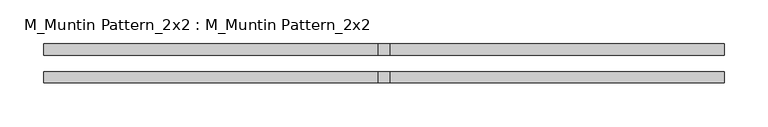
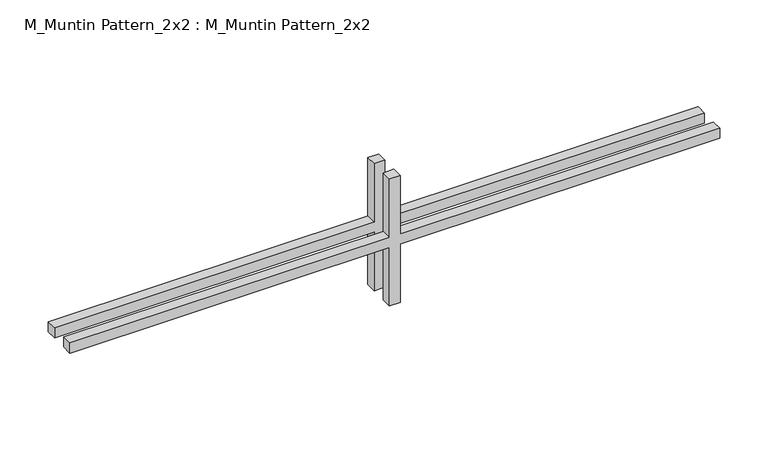
"""IFC4 building model written with IfcOpenShell, lengths in millimetres: proxy geometry, M_Muntin Pattern_2x2 : M_Muntin Pattern_2x2."""

from ifc_helpers import new_model, si_unit, frame, origin, place, context, project, spatial, polyline, outline, extrude, source, transform, mapped, element, save


def m_muntin_pattern_2x2_m_muntin_pattern_2x2_3c44882e(model_context):
    return source(origin(), model_context, "Body", "SweptSolid", [
        extrude(outline(polyline([(86.5, -6.35), (86.5, -387.35), (73.8, -387.35), (73.8, -6.35), (0.0, -6.35), (0.0, 6.35), (73.8, 6.35), (73.8, 387.35), (86.5, 387.35), (86.5, 6.35), (160.3, 6.35), (160.3, -6.35), (86.5, -6.35)])), frame((0.0, 9.525, 0.0), z_axis=(0.0, 1.0, 0.0), x_axis=(0.0, 0.0, 1.0)), (0.0, 0.0, 1.0), 12.7),
        extrude(outline(polyline([(86.5, -6.35), (86.5, -387.35), (73.8, -387.35), (73.8, -6.35), (0.0, -6.35), (0.0, 6.35), (73.8, 6.35), (73.8, 387.35), (86.5, 387.35), (86.5, 6.35), (160.3, 6.35), (160.3, -6.35), (86.5, -6.35)])), frame((0.0, -22.225, 0.0), z_axis=(0.0, 1.0, 0.0), x_axis=(0.0, 0.0, 1.0)), (0.0, 0.0, 1.0), 12.7),
    ])


if __name__ == "__main__":
    model = new_model("IFC4")
    model_context = context("Model", 3, world=origin())
    ifc_project = project(units=[si_unit("LENGTHUNIT", "METRE", prefix="MILLI")], contexts=[model_context])
    site = spatial("IfcSite", under=ifc_project)
    building = spatial("IfcBuilding", under=site)
    placement = place(None, origin())
    m_muntin_pattern_2x2_m_muntin_pattern_2x2_shape = m_muntin_pattern_2x2_m_muntin_pattern_2x2_3c44882e(model_context)
    element("IfcBuildingElementProxy", 1, Name="M_Muntin Pattern_2x2 : M_Muntin Pattern_2x2", ObjectType="M_Muntin Pattern_2x2 : M_Muntin Pattern_2x2", at=placement, inside=building, context=model_context, shape_type="MappedRepresentation", body=[
        mapped(m_muntin_pattern_2x2_m_muntin_pattern_2x2_shape, transform((0.0, 0.0, 0.0), x_axis=(1.0, 0.0, 0.0), y_axis=(0.0, 1.0, 0.0), z_axis=(0.0, 0.0, 1.0))),
    ])
    save(model, "model.ifc")

# Revit data of these elements
# Type "M_Muntin Pattern_2x2 : M_Muntin Pattern_2x2"
#   Width [instance default] = 3' - 11.24409"
#   Thickness = 0' - 0 1/2"
#   Height [instance default] = 3' - 11.24409"
#   Distance = 0' - 0 3/4"
#   Interior Material [instance default] = none
#   Exterior Material [instance default] = none
#   Default Elevation = 0
# Element 1 (IfcBuildingElementProxy, "M_Muntin Pattern_2x2 : M_Muntin Pattern_2x2")
#   Width = 2' - 6 1/2"
#   Height = 0' - 6.31102"
#   Interior Material = Wood - Stained
#   Exterior Material = Clad - White
#   Materials on its faces: "Clad - White", "Wood - Stained"
# Materials
#   "Clad - White": class "Wood", colour RGB 242 242 238, transparency 0, Cost = 0
#   "Wood - Stained": class "Wood", colour RGB 224 178 126, transparency 0, Cost = 0
